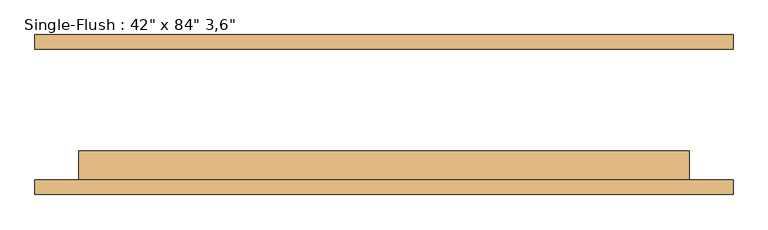
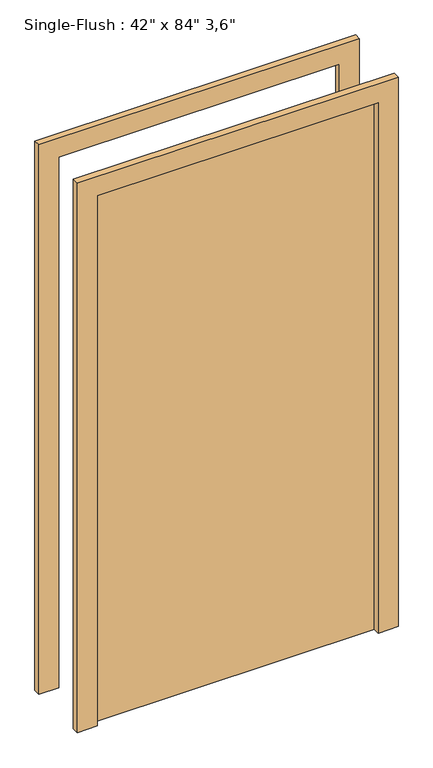
"""IFC4 building model written with IfcOpenShell, lengths in millimetres: door geometry."""

from ifc_helpers import new_model, si_unit, frame, origin, origin_with_axes, place, context, project, spatial, polyline, outline, extrude, source, transform, mapped, element, save


def door_0848dd25(model_context):
    return source(origin(), model_context, "Body", "SweptSolid", [
        extrude(outline(polyline([(2209.8, -609.6), (0.0, -609.6), (0.0, -533.4), (2133.6, -533.4), (2133.6, 533.4), (0.0, 533.4), (0.0, 609.6), (2209.8, 609.6), (2209.8, -609.6)])), frame((0.0, -139.7, 0.0), z_axis=(0.0, 1.0, 0.0), x_axis=(0.0, 0.0, 1.0)), (0.0, 0.0, 1.0), 25.4),
        extrude(outline(polyline([(2209.8, 609.6), (2209.8, -609.6), (0.0, -609.6), (0.0, -533.4), (2133.6, -533.4), (2133.6, 533.4), (0.0, 533.4), (0.0, 609.6), (2209.8, 609.6)])), frame((0.0, 114.3, 0.0), z_axis=(0.0, 1.0, 0.0), x_axis=(0.0, 0.0, 1.0)), (0.0, 0.0, 1.0), 25.4),
        extrude(outline(polyline([(533.4, -63.5), (533.4, -114.3), (-533.4, -114.3), (-533.4, -63.5), (533.4, -63.5)])), origin_with_axes(), (0.0, 0.0, 1.0), 2133.6),
    ])


if __name__ == "__main__":
    model = new_model("IFC4")
    model_context = context("Model", 3, world=origin())
    ifc_project = project(units=[si_unit("LENGTHUNIT", "METRE", prefix="MILLI")], contexts=[model_context])
    site = spatial("IfcSite", under=ifc_project)
    building = spatial("IfcBuilding", under=site)
    placement = place(None, origin())
    door_shape = door_0848dd25(model_context)
    element("IfcDoor", 1, ObjectType="Single-Flush : 42\" x 84\" 3,6\"", at=placement, inside=building, context=model_context, shape_type="MappedRepresentation", body=[
        mapped(door_shape, transform((0.0, 0.0, 0.0), x_axis=(1.0, 0.0, 0.0), y_axis=(0.0, 1.0, 0.0), z_axis=(0.0, 0.0, 1.0))),
    ])
    save(model, "model.ifc")

# Revit data of these elements
# Type "Single-Flush : 42\" x 84\" 3,6\""
#   Type Mark = "8"
#   Assembly Code = "C1020"
#   Thickness = 0' - 2"
#   Height = 7' - 0"
#   Trim Projection Ext = 0' - 1"
#   Trim Projection Int = 0' - 1"
#   Trim Width = 0' - 3"
#   Width = 3' - 6"
#   Door Material = Door - Panel
#   Frame Material = Door - Frame
#   Function = (empty or 0)
#   Wall Closure = (empty or 0)
# Element 1 (IfcDoor, "Single-Flush : 42\" x 84\" 3,6\"")
#   Materials on its faces: "Door - Frame", "Door - Panel"
# Materials
#   "Door - Panel": class "Wood", colour RGB 114 82 51, transparency 0
#   "Door - Frame": colour RGB 153 76 43, transparency 0
